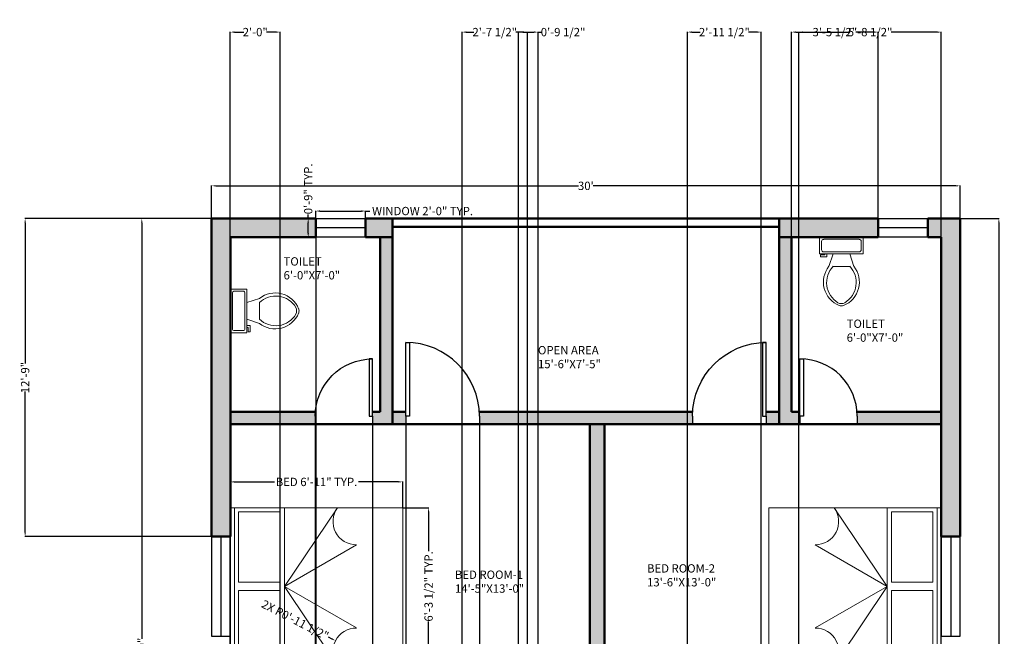
# Model space of a CAD drawing. Units: inches. Extents: x 2430 to 2930, y 1715 to 2575.
# Tile 4 of 4: x 2433 to 2907, y 2278 to 2575. Entities that reach past the tile are written whole.
import ezdxf

# ---------------------------------------------------------------- set-up
doc = ezdxf.new("R2010")
doc.units = ezdxf.units.IN
for name, color, linetype, lineweight in [('A-ANNO-DIMS', 2, 'Continuous', 18), ('A-AREA-IDEN', 130, 'Continuous', 18), ('A-FLOR-FIXT', 200, 'Continuous', 18), ('A-FURN', 200, 'Continuous', 18), ('A-WALL', 7, 'Continuous', 50), ('A-WALL-PATT', 251, 'Continuous', 13), ('DOOR', 224, 'Continuous', 25), ('win', 170, 'Continuous', 25)]:
    doc.layers.add(name, color=color, linetype=linetype, lineweight=lineweight)
doc.styles.get("Standard").update_dxf_attribs({"font": 'arial.ttf', "height": 4})
doc.dimstyles.get("Standard").update_dxf_attribs({"dimtxt": 4, "dimasz": 2, "dimexe": 0.18, "dimexo": 0.0625, "dimgap": 0.09, "dimtad": 0, "dimzin": 0, "dimdsep": 46, "dimlunit": 3, "dimtxsty": 'Standard', "dimcen": 0.09, "dimadec": 0, "dimazin": 0, "dimtfac": 1, "dimtofl": 0, "dimtmove": 0, "dimatfit": 3, "dimfxl": 1, "dimtolj": 1, "dimtzin": 0, "dimarcsym": 0})

# ---------------------------------------------------------------- blocks, each defined once
blk = doc.blocks.new('*U4')
for p, q in [((0, 0), (0, -100)), ((700, 0), (700, -100))]:
    blk.add_line(p, q)
blk.add_lwpolyline([(0, 0), (0, 700), (43.75, 700), (43.75, 0)], close=True)
blk.add_arc((0, 0), 700, 0, 90)
blk = doc.blocks.new('*U7')
for p, q in [((0, 0), (0, -100)), ((900, 0), (900, -100))]:
    blk.add_line(p, q)
blk.add_lwpolyline([(0, 0), (0, 900), (43.75, 900), (43.75, 0)], close=True)
blk.add_arc((0, 0), 900, 0, 90)
blk = doc.blocks.new('*U9')
for p, q in [((241, -152), (241, -51)), ((-254, -216), (-203, -216)), ((-254, -241), (-254, -216)), ((-203, -216), (-203, -203)), ((-178, -203), (-178, -241)), ((-102, -203), (-152, -356)), ((102, -203), (152, -356)), ((-178, -241), (-254, -241)), ((102, -356), (-102, -356))]:
    blk.add_line(p, q)
blk.add_lwpolyline([(267, -203), (267, 0), (-267, 0), (-267, -203)], close=True)
for points in [[(-241, -51), (-241, -152)], [(216, -25), (-216, -25)], [(-216, -178), (216, -178)]]:
    blk.add_lwpolyline(points)
for centre, radius, start, end in [((-219, -48), 22.5, 81.8699, 188.1301), ((219, -48), 22.5, 351.8699, 98.1301), ((-219, -156), 22.5, 171.8699, 278.1301), ((219, -156), 22.5, 261.8699, 8.1301), ((89, -548), 309, 141.4691, 247.9714), ((107, -554), 288, 136.3677, 238.9468), ((-89, -548), 309, 292.0284, 38.5307), ((-107, -554), 288, 301.053, 43.6321), ((0, -708), 102, 245.7318, 294.2682), ((0, -737), 102, 254.8605, 285.1395)]:
    blk.add_arc(centre, radius, start, end)
blk = doc.blocks.new('NEW BED')
for p, q in [((-75.7, 82.92), (0, 82.92)), ((-75.7, 0), (-75.7, 82.92)), ((-75.7, 80.92), (0, 80.92)), ((0, 82.92), (0, 0)), ((-73.7, 78.92), (-39.85, 78.92)), ((-73.7, 58.92), (-73.7, 78.92)), ((-39.85, 58.92), (-39.85, 78.92)), ((-35.85, 78.92), (-2, 78.92)), ((-35.85, 58.92), (-35.85, 78.92)), ((-2, 78.92), (-2, 58.92)), ((-75.7, 56.92), (0, 56.92)), ((-37.85, 56.92), (-75.7, 31.45)), ((-73.7, 58.92), (-39.85, 58.92)), ((-37.85, 56.92), (-57.85, 22.27)), ((-37.85, 56.92), (0, 31.45)), ((-37.85, 56.92), (-17.84, 22.27)), ((-35.85, 58.92), (-2, 58.92)), ((0, 0), (-75.7, 0))]:
    blk.add_line(p, q)
for centre, start, end in [((-69.14, 22.27), 0, 125.5497), ((-6.56, 22.27), 54.4503, 180)]:
    blk.add_arc(centre, 11.28, start, end)
blk = doc.blocks.new('*D11')
at = {"layer": 'A-ANNO-DIMS', "color": 0, "lineweight": -2, "transparency": 16777216}
for p, q in [((2525.62, 2479.52), (2525.62, 2495.36)), ((2527.62, 2495.18), (2702.14, 2495.18)), ((2883.62, 2495.18), (2709.1, 2495.18)), ((2885.62, 2479.52), (2885.62, 2495.36))]:
    blk.add_line(p, q, dxfattribs=at)
at = {"layer": 'A-ANNO-DIMS', "color": 0, "transparency": 16777216}
for points in [[(2527.62, 2495.51), (2527.62, 2494.85), (2525.62, 2495.18)], [(2883.62, 2495.51), (2883.62, 2494.85), (2885.62, 2495.18)]]:
    blk.add_solid(points, dxfattribs=at)
at = {"layer": 'Defpoints', "color": 0, "transparency": 16777216}
for p in [(2885.62, 2495.18), (2525.62, 2479.45), (2885.62, 2479.45)]:
    blk.add_point(p, dxfattribs=at)
at = {"layer": 'A-ANNO-DIMS', "color": 0, "transparency": 16777216, "insert": (2705.62, 2495.18), "char_height": 4, "attachment_point": 5}
blk.add_mtext("\\A1;30'", dxfattribs=at)
blk = doc.blocks.new('*D12')
at = {"layer": 'A-ANNO-DIMS', "color": 0, "lineweight": -2, "transparency": 16777216}
for p, q in [((2885.68, 2479.45), (2904.48, 2479.45)), ((2904.3, 2477.45), (2904.3, 2122.95)), ((2904.3, 1761.45), (2904.3, 2115.96)), ((2885.68, 1759.45), (2904.48, 1759.45))]:
    blk.add_line(p, q, dxfattribs=at)
at = {"layer": 'A-ANNO-DIMS', "color": 0, "transparency": 16777216}
for points in [[(2903.96, 2477.45), (2904.63, 2477.45), (2904.3, 2479.45)], [(2903.96, 1761.45), (2904.63, 1761.45), (2904.3, 1759.45)]]:
    blk.add_solid(points, dxfattribs=at)
at = {"layer": 'Defpoints', "color": 0, "transparency": 16777216}
for p in [(2885.62, 2479.45), (2885.62, 1759.45), (2904.3, 1759.45)]:
    blk.add_point(p, dxfattribs=at)
at = {"layer": 'A-ANNO-DIMS', "color": 0, "transparency": 16777216, "insert": (2904.3, 2119.45), "char_height": 4, "attachment_point": 5, "rotation": 90}
blk.add_mtext("\\A1;60'", dxfattribs=at)
blk = doc.blocks.new('*D13')
at = {"layer": 'A-ANNO-DIMS', "color": 0, "lineweight": -2, "transparency": 16777216}
for p, q in [((2525.56, 2479.45), (2491.85, 2479.45)), ((2492.03, 2477.45), (2492.03, 2277.3)), ((2492.03, 2055.45), (2492.03, 2255.61)), ((2534.56, 2053.45), (2491.85, 2053.45))]:
    blk.add_line(p, q, dxfattribs=at)
at = {"layer": 'A-ANNO-DIMS', "color": 0, "transparency": 16777216}
for points in [[(2491.69, 2477.45), (2492.36, 2477.45), (2492.03, 2479.45)], [(2491.69, 2055.45), (2492.36, 2055.45), (2492.03, 2053.45)]]:
    blk.add_solid(points, dxfattribs=at)
at = {"layer": 'Defpoints', "color": 0, "transparency": 16777216}
for p in [(2525.62, 2479.45), (2492.03, 2053.45), (2534.62, 2053.45)]:
    blk.add_point(p, dxfattribs=at)
at = {"layer": 'A-ANNO-DIMS', "color": 0, "transparency": 16777216, "insert": (2492.03, 2266.45), "char_height": 4, "attachment_point": 5, "rotation": 90}
blk.add_mtext('\\A1;35\'-6.00"', dxfattribs=at)
blk = doc.blocks.new('WIN-48IN')
blk.add_line((0, 4.5), (48, 4.5))
blk.add_lwpolyline([(0, 9), (48, 9), (48, 0), (0, 0)], close=True)
blk = doc.blocks.new('WIN-24IN')
blk.add_line((24, 4.5), (0, 4.5))
blk.add_lwpolyline([(0, 9), (24, 9), (24, 0), (0, 0)], close=True)
blk = doc.blocks.new('*D19')
at = {"layer": 'A-ANNO-DIMS', "color": 0, "lineweight": -2, "transparency": 16777216}
for p, q in [((2575.68, 2479.52), (2575.68, 2483.23)), ((2577.68, 2483.05), (2597.68, 2483.05)), ((2599.68, 2479.52), (2599.68, 2483.23)), ((2599.68, 2483.05), (2601.68, 2483.05))]:
    blk.add_line(p, q, dxfattribs=at)
at = {"layer": 'A-ANNO-DIMS', "color": 0, "transparency": 16777216}
for points in [[(2577.68, 2483.39), (2577.68, 2482.72), (2575.68, 2483.05)], [(2597.68, 2483.39), (2597.68, 2482.72), (2599.68, 2483.05)]]:
    blk.add_solid(points, dxfattribs=at)
at = {"layer": 'Defpoints', "color": 0, "transparency": 16777216}
for p in [(2599.68, 2483.05), (2575.68, 2479.45), (2599.68, 2479.45)]:
    blk.add_point(p, dxfattribs=at)
at = {"layer": 'A-ANNO-DIMS', "color": 0, "transparency": 16777216, "insert": (2627.08, 2483.05), "char_height": 4, "attachment_point": 5}
blk.add_mtext('\\A1;WINDOW 2\'-0" TYP.', dxfattribs=at)
blk = doc.blocks.new('*D20')
at = {"layer": 'A-ANNO-DIMS', "color": 0, "lineweight": -2, "transparency": 16777216}
for p, q in [((2575.62, 2479.45), (2571.9, 2479.45)), ((2572.08, 2479.45), (2572.08, 2481.45)), ((2572.08, 2472.45), (2572.08, 2477.45)), ((2575.62, 2470.45), (2571.9, 2470.45))]:
    blk.add_line(p, q, dxfattribs=at)
at = {"layer": 'A-ANNO-DIMS', "color": 0, "transparency": 16777216}
for points in [[(2571.75, 2477.45), (2572.42, 2477.45), (2572.08, 2479.45)], [(2571.75, 2472.45), (2572.42, 2472.45), (2572.08, 2470.45)]]:
    blk.add_solid(points, dxfattribs=at)
at = {"layer": 'Defpoints', "color": 0, "transparency": 16777216}
for p in [(2572.08, 2479.45), (2575.68, 2479.45), (2575.68, 2470.45)]:
    blk.add_point(p, dxfattribs=at)
at = {"layer": 'A-ANNO-DIMS', "color": 0, "transparency": 16777216, "insert": (2572.08, 2493.73), "char_height": 4, "attachment_point": 5, "rotation": 90}
blk.add_mtext('\\A1;0\'-9" TYP.', dxfattribs=at)
blk = doc.blocks.new('*D21')
at = {"layer": 'A-ANNO-DIMS', "color": 0, "lineweight": -2, "transparency": 16777216}
for p, q in [((2534.62, 2340.36), (2534.62, 2352.92)), ((2536.62, 2352.74), (2555.81, 2352.74)), ((2615.54, 2352.74), (2596.35, 2352.74)), ((2617.54, 2340.36), (2617.54, 2352.92))]:
    blk.add_line(p, q, dxfattribs=at)
at = {"layer": 'A-ANNO-DIMS', "color": 0, "transparency": 16777216}
for points in [[(2536.62, 2353.07), (2536.62, 2352.41), (2534.62, 2352.74)], [(2615.54, 2353.07), (2615.54, 2352.41), (2617.54, 2352.74)]]:
    blk.add_solid(points, dxfattribs=at)
at = {"layer": 'Defpoints', "color": 0, "transparency": 16777216}
for p in [(2534.62, 2352.74), (2534.62, 2340.3), (2617.54, 2340.3)]:
    blk.add_point(p, dxfattribs=at)
at = {"layer": 'A-ANNO-DIMS', "color": 0, "transparency": 16777216, "insert": (2576.08, 2352.74), "char_height": 4, "attachment_point": 5}
blk.add_mtext('\\A1;BED 6\'-11" TYP.', dxfattribs=at)
blk = doc.blocks.new('*D22')
at = {"layer": 'A-ANNO-DIMS', "color": 0, "lineweight": -2, "transparency": 16777216}
for p, q in [((2617.61, 2340.3), (2630.16, 2340.3)), ((2629.98, 2338.3), (2629.98, 2319.41)), ((2629.98, 2266.6), (2629.98, 2285.5)), ((2617.61, 2264.6), (2630.16, 2264.6))]:
    blk.add_line(p, q, dxfattribs=at)
at = {"layer": 'A-ANNO-DIMS', "color": 0, "transparency": 16777216}
for points in [[(2629.65, 2338.3), (2630.31, 2338.3), (2629.98, 2340.3)], [(2629.65, 2266.6), (2630.31, 2266.6), (2629.98, 2264.6)]]:
    blk.add_solid(points, dxfattribs=at)
at = {"layer": 'Defpoints', "color": 0, "transparency": 16777216}
for p in [(2617.54, 2340.3), (2629.98, 2340.3), (2617.54, 2264.6)]:
    blk.add_point(p, dxfattribs=at)
at = {"layer": 'A-ANNO-DIMS', "color": 0, "transparency": 16777216, "insert": (2629.98, 2302.45), "char_height": 4, "attachment_point": 5, "rotation": 90}
blk.add_mtext('\\A1;6\'-3 1/2" TYP.', dxfattribs=at)
blk = doc.blocks.new('*D25')
at = {"layer": 'A-ANNO-DIMS', "color": 0, "lineweight": -2, "transparency": 16777216}
for p, q in [((2754.56, 2067.12), (2754.56, 2569.33)), ((2756.56, 2569.15), (2760.62, 2569.15)), ((2787.99, 2569.15), (2783.93, 2569.15)), ((2789.99, 2067.12), (2789.99, 2569.33))]:
    blk.add_line(p, q, dxfattribs=at)
at = {"layer": 'A-ANNO-DIMS', "color": 0, "transparency": 16777216}
for points in [[(2756.56, 2569.49), (2756.56, 2568.82), (2754.56, 2569.15)], [(2787.99, 2569.49), (2787.99, 2568.82), (2789.99, 2569.15)]]:
    blk.add_solid(points, dxfattribs=at)
at = {"layer": 'Defpoints', "color": 0, "transparency": 16777216}
for p in [(2789.99, 2569.15), (2754.56, 2067.05), (2789.99, 2067.05)]:
    blk.add_point(p, dxfattribs=at)
at = {"layer": 'A-ANNO-DIMS', "color": 0, "transparency": 16777216, "insert": (2772.27, 2569.15), "char_height": 4, "attachment_point": 5}
blk.add_mtext('\\A1;2\'-11 1/2"', dxfattribs=at)
blk = doc.blocks.new('*D30')
at = {"layer": 'A-ANNO-DIMS', "color": 0, "lineweight": -2, "transparency": 16777216}
for p, q in [((2534.62, 2470.39), (2534.62, 1720.57)), ((2575.68, 2470.39), (2575.68, 1720.57)), ((2536.62, 1720.75), (2549.75, 1720.75)), ((2573.68, 1720.75), (2560.56, 1720.75))]:
    blk.add_line(p, q, dxfattribs=at)
at = {"layer": 'A-ANNO-DIMS', "color": 0, "transparency": 16777216}
for points in [[(2536.62, 1721.09), (2536.62, 1720.42), (2534.62, 1720.75)], [(2573.68, 1721.09), (2573.68, 1720.42), (2575.68, 1720.75)]]:
    blk.add_solid(points, dxfattribs=at)
at = {"layer": 'Defpoints', "color": 0, "transparency": 16777216}
for p in [(2534.62, 2470.45), (2575.68, 2470.45), (2575.68, 1720.75)]:
    blk.add_point(p, dxfattribs=at)
at = {"layer": 'A-ANNO-DIMS', "color": 0, "transparency": 16777216, "insert": (2555.15, 1720.75), "char_height": 4, "attachment_point": 5}
blk.add_mtext('\\A1;3\'-5"', dxfattribs=at)
blk = doc.blocks.new('*D31')
at = {"layer": 'A-ANNO-DIMS', "color": 0, "lineweight": -2, "transparency": 16777216}
for p, q in [((2804.62, 2470.52), (2804.62, 2569.33)), ((2806.62, 2569.15), (2815.33, 2569.15)), ((2844.18, 2569.15), (2835.46, 2569.15)), ((2846.18, 2470.52), (2846.18, 2569.33))]:
    blk.add_line(p, q, dxfattribs=at)
at = {"layer": 'A-ANNO-DIMS', "color": 0, "transparency": 16777216}
for points in [[(2806.62, 2569.49), (2806.62, 2568.82), (2804.62, 2569.15)], [(2844.18, 2569.49), (2844.18, 2568.82), (2846.18, 2569.15)]]:
    blk.add_solid(points, dxfattribs=at)
at = {"layer": 'Defpoints', "color": 0, "transparency": 16777216}
for p in [(2846.18, 2569.15), (2804.62, 2470.45), (2846.18, 2470.45)]:
    blk.add_point(p, dxfattribs=at)
at = {"layer": 'A-ANNO-DIMS', "color": 0, "transparency": 16777216, "insert": (2825.4, 2569.15), "char_height": 4, "attachment_point": 5}
blk.add_mtext('\\A1;3\'-5 1/2"', dxfattribs=at)
blk = doc.blocks.new('*D32')
at = {"layer": 'A-ANNO-DIMS', "color": 0, "lineweight": -2, "transparency": 16777216}
for p, q in [((2525.56, 2479.45), (2435.74, 2479.45)), ((2435.92, 2477.45), (2435.92, 2409.72)), ((2435.92, 2328.45), (2435.92, 2396.18)), ((2525.56, 2326.45), (2435.74, 2326.45))]:
    blk.add_line(p, q, dxfattribs=at)
at = {"layer": 'A-ANNO-DIMS', "color": 0, "transparency": 16777216}
for points in [[(2435.59, 2477.45), (2436.25, 2477.45), (2435.92, 2479.45)], [(2435.59, 2328.45), (2436.25, 2328.45), (2435.92, 2326.45)]]:
    blk.add_solid(points, dxfattribs=at)
at = {"layer": 'Defpoints', "color": 0, "transparency": 16777216}
for p in [(2525.62, 2479.45), (2435.92, 2326.45), (2525.62, 2326.45)]:
    blk.add_point(p, dxfattribs=at)
at = {"layer": 'A-ANNO-DIMS', "color": 0, "transparency": 16777216, "insert": (2435.92, 2402.95), "char_height": 4, "attachment_point": 5, "rotation": 90}
blk.add_mtext('\\A1;12\'-9"', dxfattribs=at)
blk = doc.blocks.new('*D39')
at = {"layer": 'A-ANNO-DIMS', "color": 0, "lineweight": -2, "transparency": 16777216}
for p, q in [((2808.12, 1840.52), (2808.12, 2569.33)), ((2810.12, 2569.15), (2832.3, 2569.15)), ((2874.62, 2569.15), (2852.44, 2569.15)), ((2876.62, 1840.52), (2876.62, 2569.33))]:
    blk.add_line(p, q, dxfattribs=at)
at = {"layer": 'A-ANNO-DIMS', "color": 0, "transparency": 16777216}
for points in [[(2810.12, 2569.49), (2810.12, 2568.82), (2808.12, 2569.15)], [(2874.62, 2569.49), (2874.62, 2568.82), (2876.62, 2569.15)]]:
    blk.add_solid(points, dxfattribs=at)
at = {"layer": 'Defpoints', "color": 0, "transparency": 16777216}
for p in [(2876.62, 2569.15), (2808.12, 1840.45), (2876.62, 1840.45)]:
    blk.add_point(p, dxfattribs=at)
at = {"layer": 'A-ANNO-DIMS', "color": 0, "transparency": 16777216, "insert": (2842.37, 2569.15), "char_height": 4, "attachment_point": 5}
blk.add_mtext('\\A1;5\'-8 1/2"', dxfattribs=at)
blk = doc.blocks.new('*D42')
at = {"layer": 'A-ANNO-DIMS', "color": 0, "lineweight": -2, "transparency": 16777216}
for p, q in [((2646.07, 2053.52), (2646.07, 2569.33)), ((2648.07, 2569.15), (2651.72, 2569.15)), ((2675.57, 2569.15), (2671.92, 2569.15)), ((2677.57, 2053.52), (2677.57, 2569.33))]:
    blk.add_line(p, q, dxfattribs=at)
at = {"layer": 'A-ANNO-DIMS', "color": 0, "transparency": 16777216}
for points in [[(2648.07, 2569.49), (2648.07, 2568.82), (2646.07, 2569.15)], [(2675.57, 2569.49), (2675.57, 2568.82), (2677.57, 2569.15)]]:
    blk.add_solid(points, dxfattribs=at)
at = {"layer": 'Defpoints', "color": 0, "transparency": 16777216}
for p in [(2677.57, 2569.15), (2646.07, 2053.45), (2677.57, 2053.45)]:
    blk.add_point(p, dxfattribs=at)
at = {"layer": 'A-ANNO-DIMS', "color": 0, "transparency": 16777216, "insert": (2661.82, 2569.15), "char_height": 4, "attachment_point": 5}
blk.add_mtext('\\A1;2\'-7 1/2"', dxfattribs=at)
blk = doc.blocks.new('*D43')
at = {"layer": 'A-ANNO-DIMS', "color": 0, "lineweight": -2, "transparency": 16777216}
for p, q in [((2673.24, 1966.52), (2673.24, 2569.33)), ((2675.24, 2569.15), (2680.62, 2569.15)), ((2682.62, 1966.52), (2682.62, 2569.33)), ((2682.62, 2569.15), (2684.62, 2569.15))]:
    blk.add_line(p, q, dxfattribs=at)
at = {"layer": 'A-ANNO-DIMS', "color": 0, "transparency": 16777216}
for points in [[(2675.24, 2569.49), (2675.24, 2568.82), (2673.24, 2569.15)], [(2680.62, 2569.49), (2680.62, 2568.82), (2682.62, 2569.15)]]:
    blk.add_solid(points, dxfattribs=at)
at = {"layer": 'Defpoints', "color": 0, "transparency": 16777216}
for p in [(2682.62, 2569.15), (2673.24, 1966.45), (2682.62, 1966.45)]:
    blk.add_point(p, dxfattribs=at)
at = {"layer": 'A-ANNO-DIMS', "color": 0, "transparency": 16777216, "insert": (2694.69, 2569.15), "char_height": 4, "attachment_point": 5}
blk.add_mtext('\\A1;0\'-9 1/2"', dxfattribs=at)
blk = doc.blocks.new('*D45')
at = {"layer": 'A-ANNO-DIMS', "color": 0, "lineweight": -2, "transparency": 16777216}
for p, q in [((2619.01, 2380.39), (2619.01, 1720.57)), ((2654.44, 2380.39), (2654.44, 1720.57)), ((2621.01, 1720.75), (2625.07, 1720.75)), ((2652.44, 1720.75), (2648.38, 1720.75))]:
    blk.add_line(p, q, dxfattribs=at)
at = {"layer": 'A-ANNO-DIMS', "color": 0, "transparency": 16777216}
for points in [[(2621.01, 1721.09), (2621.01, 1720.42), (2619.01, 1720.75)], [(2652.44, 1721.09), (2652.44, 1720.42), (2654.44, 1720.75)]]:
    blk.add_solid(points, dxfattribs=at)
at = {"layer": 'Defpoints', "color": 0, "transparency": 16777216}
for p in [(2619.01, 2380.45), (2654.44, 2380.45), (2654.44, 1720.75)]:
    blk.add_point(p, dxfattribs=at)
at = {"layer": 'A-ANNO-DIMS', "color": 0, "transparency": 16777216, "insert": (2636.72, 1720.75), "char_height": 4, "attachment_point": 5}
blk.add_mtext('\\A1;2\'-11 1/2"', dxfattribs=at)
blk = doc.blocks.new('*D46')
at = {"layer": 'A-ANNO-DIMS', "color": 0, "lineweight": -2, "transparency": 16777216}
for p, q in [((2575.5, 2380.39), (2575.5, 1720.57)), ((2603.06, 2380.39), (2603.06, 1720.57)), ((2577.5, 1720.75), (2579.18, 1720.75)), ((2601.06, 1720.75), (2599.38, 1720.75))]:
    blk.add_line(p, q, dxfattribs=at)
at = {"layer": 'A-ANNO-DIMS', "color": 0, "transparency": 16777216}
for points in [[(2577.5, 1721.09), (2577.5, 1720.42), (2575.5, 1720.75)], [(2601.06, 1721.09), (2601.06, 1720.42), (2603.06, 1720.75)]]:
    blk.add_solid(points, dxfattribs=at)
at = {"layer": 'Defpoints', "color": 0, "transparency": 16777216}
for p in [(2575.5, 2380.45), (2603.06, 2380.45), (2603.06, 1720.75)]:
    blk.add_point(p, dxfattribs=at)
at = {"layer": 'A-ANNO-DIMS', "color": 0, "transparency": 16777216, "insert": (2589.28, 1720.75), "char_height": 4, "attachment_point": 5}
blk.add_mtext('\\A1;2\'-3 1/2"', dxfattribs=at)
blk = doc.blocks.new('*D49')
at = {"layer": 'A-ANNO-DIMS', "color": 0, "lineweight": -2, "transparency": 16777216}
for p, q in [((2534.62, 2062.52), (2534.62, 2569.33)), ((2536.62, 2569.15), (2541.18, 2569.15)), ((2556.62, 2569.15), (2552.06, 2569.15)), ((2558.62, 2062.52), (2558.62, 2569.33))]:
    blk.add_line(p, q, dxfattribs=at)
at = {"layer": 'A-ANNO-DIMS', "color": 0, "transparency": 16777216}
for points in [[(2536.62, 2569.49), (2536.62, 2568.82), (2534.62, 2569.15)], [(2556.62, 2569.49), (2556.62, 2568.82), (2558.62, 2569.15)]]:
    blk.add_solid(points, dxfattribs=at)
at = {"layer": 'Defpoints', "color": 0, "transparency": 16777216}
for p in [(2558.62, 2569.15), (2534.62, 2062.45), (2558.62, 2062.45)]:
    blk.add_point(p, dxfattribs=at)
at = {"layer": 'A-ANNO-DIMS', "color": 0, "transparency": 16777216, "insert": (2546.62, 2569.15), "char_height": 4, "attachment_point": 5}
blk.add_mtext('\\A1;2\'-0"', dxfattribs=at)
blk = doc.blocks.new('*D55')
at = {"layer": 'A-ANNO-DIMS', "color": 0, "lineweight": -2, "transparency": 16777216}
for p, q in [((2581.68, 2278.16), (2583.46, 2277.24)), ((2595.18, 2271.16), (2595.36, 2271.16)), ((2595.27, 2271.07), (2595.27, 2271.25))]:
    blk.add_line(p, q, dxfattribs=at)
at = {"layer": 'A-ANNO-DIMS', "color": 0, "transparency": 16777216}
blk.add_solid([(2583.61, 2277.54), (2583.31, 2276.94), (2585.24, 2276.33)], dxfattribs=at)
at = {"layer": 'Defpoints', "color": 0, "transparency": 16777216}
for p in [(2585.24, 2276.33), (2595.27, 2271.16)]:
    blk.add_point(p, dxfattribs=at)
at = {"layer": 'A-ANNO-DIMS', "color": 0, "transparency": 16777216, "insert": (2565.79, 2286.33), "char_height": 4, "attachment_point": 5, "rotation": 332.7752}
blk.add_mtext('\\A1;2X R0\'-11 1/2"', dxfattribs=at)

msp = doc.modelspace()

# ---------------------------------------------------------------- hatches: boundary and pattern name
at = {"layer": 'A-WALL-PATT'}
h = msp.add_hatch(color=256, dxfattribs=at)
h.dxf.hatch_style = 1
h.paths.add_polyline_path([(2885.621, 2479.453), (2870.176, 2479.453), (2870.176, 2470.453), (2876.621, 2470.453), (2876.621, 2326.453), (2885.621, 2326.453)])
h.paths.add_polyline_path([(2876.621, 2386.453), (2836.085, 2386.453, -0.018734), (2836.163, 2384.39), (2836.163, 2380.453), (2876.621, 2380.453)])
h.paths.add_polyline_path([(2808.604, 2384.39), (2808.604, 2386.453), (2804.621, 2386.453), (2804.621, 2470.453), (2798.621, 2470.453), (2798.621, 2380.453), (2808.604, 2380.453)])
h.paths.add_polyline_path([(2798.621, 2386.453), (2792.402, 2386.453), (2792.402, 2384.39), (2792.402, 2380.453), (2798.621, 2380.453)])
h.paths.add_polyline_path([(2846.176, 2479.453), (2798.621, 2479.453), (2798.621, 2470.453), (2846.176, 2470.453)])
h.paths.add_polyline_path([(2575.684, 2479.453), (2525.621, 2479.453), (2525.621, 2326.453), (2534.621, 2326.453), (2534.621, 2340.302), (2534.621, 2470.453), (2575.684, 2470.453)])
h.paths.add_polyline_path([(2612.621, 2470.453), (2606.621, 2470.453), (2606.621, 2386.453), (2603.056, 2386.453), (2603.056, 2384.39), (2603.056, 2380.453), (2612.621, 2380.453)])
h.paths.add_polyline_path([(2575.497, 2384.39, -0.018734), (2575.575, 2386.453), (2534.621, 2386.453), (2534.621, 2380.453), (2575.497, 2380.453)], flags=17)
h.paths.add_polyline_path([(2619.005, 2384.39), (2619.005, 2386.453), (2612.621, 2386.453), (2612.621, 2380.453), (2619.005, 2380.453)])
h.paths.add_polyline_path([(2559.006, 2447.891), (2586.987, 2447.891), (2586.987, 2462.817), (2559.006, 2462.817)], flags=9)
h.paths.add_polyline_path([(2733.475, 2300.192), (2771.068, 2300.192), (2771.068, 2315.118), (2733.475, 2315.118)], flags=9)
h.paths.add_polyline_path([(2641.061, 2297.155), (2678.654, 2297.155), (2678.654, 2312.081), (2641.061, 2312.081)], flags=9)
h = msp.add_hatch(color=256, dxfattribs=at)
h.dxf.hatch_style = 1
h.paths.add_polyline_path([(2612.621, 2479.453), (2599.684, 2479.453), (2599.684, 2470.453), (2612.621, 2470.453)])
h = msp.add_hatch(color=256, dxfattribs=at)
h.dxf.hatch_style = 1
h.paths.add_polyline_path([(2714.621, 2380.453), (2707.621, 2380.453), (2707.621, 2224.453), (2705.621, 2224.453), (2705.621, 2222.39), (2705.621, 2218.453), (2715.188, 2218.453), (2715.188, 2222.39), (2715.188, 2224.453), (2714.621, 2224.453)])
h.paths.add_polyline_path([(2756.969, 2384.39, -0.0145648), (2757.029, 2386.453), (2654.378, 2386.453, -0.0145648), (2654.438, 2384.39), (2654.438, 2380.453), (2756.969, 2380.453)])

# ---------------------------------------------------------------- linework, layer by layer
at = {"layer": 'A-WALL'}
for p, q in [((2575.684, 2470.453), (2575.684, 2479.453)), ((2599.684, 2470.453), (2599.684, 2479.453)), ((2612.621, 2470.453), (2612.621, 2479.453)), ((2798.621, 2470.453), (2798.621, 2479.453)), ((2846.176, 2470.453), (2846.176, 2479.453)), ((2870.176, 2470.453), (2870.176, 2479.453)), ((2612.621, 2475.453), (2798.621, 2475.453)), ((2534.621, 2470.453), (2575.684, 2470.453)), ((2534.621, 2326.453), (2534.621, 2470.453)), ((2599.684, 2470.453), (2612.621, 2470.453)), ((2606.621, 2386.453), (2606.621, 2470.453)), ((2612.621, 2380.453), (2612.621, 2470.453)), ((2798.621, 2470.453), (2798.621, 2380.453)), ((2798.621, 2470.453), (2846.176, 2470.453)), ((2804.621, 2470.453), (2804.621, 2386.453)), ((2870.176, 2470.453), (2876.621, 2470.453)), ((2876.621, 2470.453), (2876.621, 2326.453)), ((2534.621, 2386.453), (2575.575, 2386.453)), ((2603.056, 2386.453), (2606.621, 2386.453)), ((2612.621, 2386.453), (2619.005, 2386.453)), ((2654.378, 2386.453), (2757.029, 2386.453)), ((2792.402, 2386.453), (2798.621, 2386.453)), ((2804.621, 2386.453), (2808.604, 2386.453)), ((2836.085, 2386.453), (2876.621, 2386.453)), ((2534.621, 2380.453), (2876.621, 2380.453)), ((2707.621, 2224.453), (2707.621, 2380.453)), ((2714.621, 2224.453), (2714.621, 2380.453)), ((2534.621, 2326.453), (2525.621, 2326.453)), ((2876.621, 2326.453), (2885.621, 2326.453))]:
    msp.add_line(p, q, dxfattribs=at)
for points in [[(2525.621, 2326.453), (2525.621, 2479.453), (2575.684, 2479.453)], [(2599.684, 2479.453), (2846.176, 2479.453)], [(2870.176, 2479.453), (2885.621, 2479.453), (2885.621, 2326.453)]]:
    msp.add_lwpolyline(points, dxfattribs=at)

# ---------------------------------------------------------------- block references
at = {"layer": 'A-FLOR-FIXT', "xscale": 0.0393700787401575, "yscale": 0.0393700787401575, "zscale": 0.0393700787401575}
msp.add_blockref('*U9', (2828.554, 2470.453), dxfattribs=at)
at = {"layer": 'A-FLOR-FIXT', "xscale": 0.0393700787401575, "yscale": 0.0393700787401575, "zscale": 0.0393700787401575, "rotation": 90}
msp.add_blockref('*U9', (2534.621, 2435.011), dxfattribs=at)
at = {"layer": 'A-FURN', "rotation": 90}
msp.add_blockref('NEW BED', (2617.543, 2340.302), dxfattribs=at)
at = {"layer": 'A-FURN', "xscale": -1, "rotation": 270}
msp.add_blockref('NEW BED', (2793.7, 2340.302), dxfattribs=at)
at = {"layer": 'DOOR', "yscale": 0.0393700787401575, "zscale": 0.0393700787401575}
for name, p, xscale in [('*U7', (2619.005, 2384.39), 0.0393700787401575), ('*U7', (2792.402, 2384.39), -0.0393700787401575), ('*U4', (2603.056, 2384.39), -0.0393700787401575), ('*U4', (2808.604, 2384.39), 0.0393700787401575)]:
    msp.add_blockref(name, p, dxfattribs=dict(at, xscale=xscale))
at = {"layer": 'win'}
for p in [(2575.684, 2470.453), (2846.175, 2470.453)]:
    msp.add_blockref('WIN-24IN', p, dxfattribs=at)
at = {"layer": 'win', "extrusion": (0, 0, -1), "zscale": -1, "rotation": 270.0000000000006}
for p in [(-2534.621, 2326.453), (-2885.621, 2326.453)]:
    msp.add_blockref('WIN-48IN', p, dxfattribs=at)

# ---------------------------------------------------------------- texts
at = {"layer": 'A-AREA-IDEN', "char_height": 4, "attachment_point": 1}
for s, width, insert in [('TOILET\\P6\'-0"X7\'-0"', 32.38136, (2560.216, 2460.829)), ('TOILET\\P6\'-0"X7\'-0"', 27.47641, (2831.106, 2430.835)), ('OPEN AREA\\P15\'-6"X7\'-5"', 53.94759, (2682.597, 2418.107)), ('BED ROOM-2\\P13\'-6"X13\'-0"', 50.90313, (2735.083, 2313.13)), ('BED ROOM-1\\P14\'-5"X13\'-0"', 34.722, (2642.669, 2310.093))]:
    msp.add_mtext_dynamic_manual_height_columns(s, width=width, gutter_width=20, heights=[0], dxfattribs=dict(at, insert=insert))

# ---------------------------------------------------------------- dimensions: what is measured, and where the dimension line sits
at = {"layer": 'A-ANNO-DIMS'}
for base, p1, p2, override, picture, middle in [((2677.568, 2569.153), (2646.072, 2053.453), (2677.568, 2053.453), {"dimdec": 1, "dimlfac": 1, "dimrnd": 0, "dimzin": 1, "dimdsep": 46, "dimlunit": 4, "dimfrac": 2}, '*D42', (2661.82, 2569.153)), ((2682.621, 2569.153), (2673.244, 1966.453), (2682.621, 1966.453), {"dimdec": 1, "dimlfac": 1, "dimrnd": 0, "dimzin": 1, "dimdsep": 46, "dimlunit": 4, "dimfrac": 2}, '*D43', (2694.688, 2569.153)), ((2789.991, 2569.153), (2754.558, 2067.055), (2789.991, 2067.055), {"dimdec": 1, "dimlfac": 1, "dimrnd": 0, "dimzin": 1, "dimdsep": 46, "dimlunit": 4, "dimfrac": 2}, '*D25', (2772.275, 2569.153)), ((2846.176, 2569.153), (2804.621, 2470.453), (2846.176, 2470.453), {"dimdec": 1, "dimlfac": 1, "dimrnd": 0, "dimzin": 1, "dimdsep": 46, "dimlunit": 4, "dimfrac": 2}, '*D31', (2825.399, 2569.153)), ((2876.621, 2569.153), (2808.121, 1840.453), (2876.621, 1840.453), {"dimdec": 1, "dimlfac": 1, "dimrnd": 0, "dimzin": 1, "dimdsep": 46, "dimlunit": 4, "dimfrac": 2}, '*D39', (2842.371, 2569.153)), ((2558.621, 2569.153), (2534.621, 2062.453), (2558.621, 2062.453), {"dimdec": 1, "dimlfac": 1, "dimrnd": 0, "dimzin": 1, "dimdsep": 46, "dimlunit": 4, "dimfrac": 2}, '*D49', (2546.621, 2569.153)), ((2885.621, 2495.18), (2525.621, 2479.453), (2885.621, 2479.453), {"dimclrd": 0, "dimclre": 0, "dimclrt": 0}, '*D11', (2705.621, 2495.18)), ((2575.684, 1720.753), (2534.621, 2470.453), (2575.684, 2470.453), {"dimdec": 1, "dimlfac": 1, "dimrnd": 0, "dimzin": 1, "dimdsep": 46, "dimlunit": 4, "dimfrac": 2}, '*D30', (2555.153, 1720.753)), ((2603.056, 1720.753), (2575.497, 2380.453), (2603.056, 2380.453), {"dimdec": 1, "dimlfac": 1, "dimrnd": 0, "dimzin": 1, "dimdsep": 46, "dimlunit": 4, "dimfrac": 2}, '*D46', (2589.277, 1720.753)), ((2654.438, 1720.753), (2619.005, 2380.453), (2654.438, 2380.453), {"dimdec": 1, "dimlfac": 1, "dimrnd": 0, "dimzin": 1, "dimdsep": 46, "dimlunit": 4, "dimfrac": 2}, '*D45', (2636.722, 1720.753))]:
    dim = msp.add_linear_dim(base=base, p1=p1, p2=p2, dimstyle='Standard', override=override, dxfattribs=at)
    dim.commit()
    dim.dimension.update_dxf_attribs({"geometry": picture, "text_midpoint": middle})
for base, p1, p2, angle, text, picture, middle in [((2572.084, 2479.453), (2575.684, 2470.453), (2575.684, 2479.453), 90, '<> TYP.', '*D20', (2572.084, 2493.734)), ((2534.621, 2352.741), (2617.543, 2340.302), (2534.621, 2340.302), 180, 'BED <> TYP.', '*D21', (2576.082, 2352.741)), ((2629.981, 2340.302), (2617.543, 2264.603), (2617.543, 2340.302), 90, '<> TYP.', '*D22', (2629.981, 2302.453))]:
    dim = msp.add_linear_dim(base=base, p1=p1, p2=p2, angle=angle, text=text, dimstyle='Standard', override={"dimdec": 1, "dimlfac": 1, "dimrnd": 0, "dimzin": 1, "dimdsep": 46, "dimlunit": 4, "dimfrac": 2}, dxfattribs=at)
    dim.commit()
    dim.dimension.update_dxf_attribs({"geometry": picture, "text_midpoint": middle})
dim = msp.add_linear_dim(base=(2599.684, 2483.053), p1=(2575.684, 2479.453), p2=(2599.684, 2479.453), text='WINDOW <> TYP.', dimstyle='Standard', override={"dimdec": 1, "dimlfac": 1, "dimrnd": 0, "dimzin": 1, "dimdsep": 46, "dimlunit": 4, "dimfrac": 2}, dxfattribs=at)
dim.commit()
dim.dimension.update_dxf_attribs({"geometry": '*D19', "text_midpoint": (2627.083, 2483.053)})
for base, p1, p2, override, picture, middle in [((2435.921, 2326.453), (2525.621, 2479.453), (2525.621, 2326.453), {"dimdec": 1, "dimlfac": 1, "dimrnd": 0, "dimzin": 1, "dimdsep": 46, "dimlunit": 4, "dimfrac": 2}, '*D32', (2435.921, 2402.953)), ((2492.026, 2053.453), (2525.621, 2479.453), (2534.621, 2053.453), {"dimclrd": 0, "dimclre": 0, "dimclrt": 0}, '*D13', (2492.026, 2266.453)), ((2904.296, 1759.453), (2885.621, 2479.453), (2885.621, 1759.453), {"dimclrd": 0, "dimclre": 0, "dimclrt": 0}, '*D12', (2904.296, 2119.453))]:
    dim = msp.add_linear_dim(base=base, p1=p1, p2=p2, angle=90, dimstyle='Standard', override=override, dxfattribs=at)
    dim.commit()
    dim.dimension.update_dxf_attribs({"geometry": picture, "text_midpoint": middle})
dim = msp.add_radius_dim(center=(2595.271, 2271.164), mpoint=(2585.237, 2276.326), text='2X <>', dimstyle='Standard', override={"dimdec": 1, "dimlfac": 1, "dimrnd": 0, "dimzin": 1, "dimdsep": 46, "dimlunit": 4, "dimfrac": 2}, dxfattribs=at)
dim.commit()
dim.dimension.update_dxf_attribs({"geometry": '*D55', "text_midpoint": (2565.793, 2286.33)})

doc.saveas('drawing.dxf')
